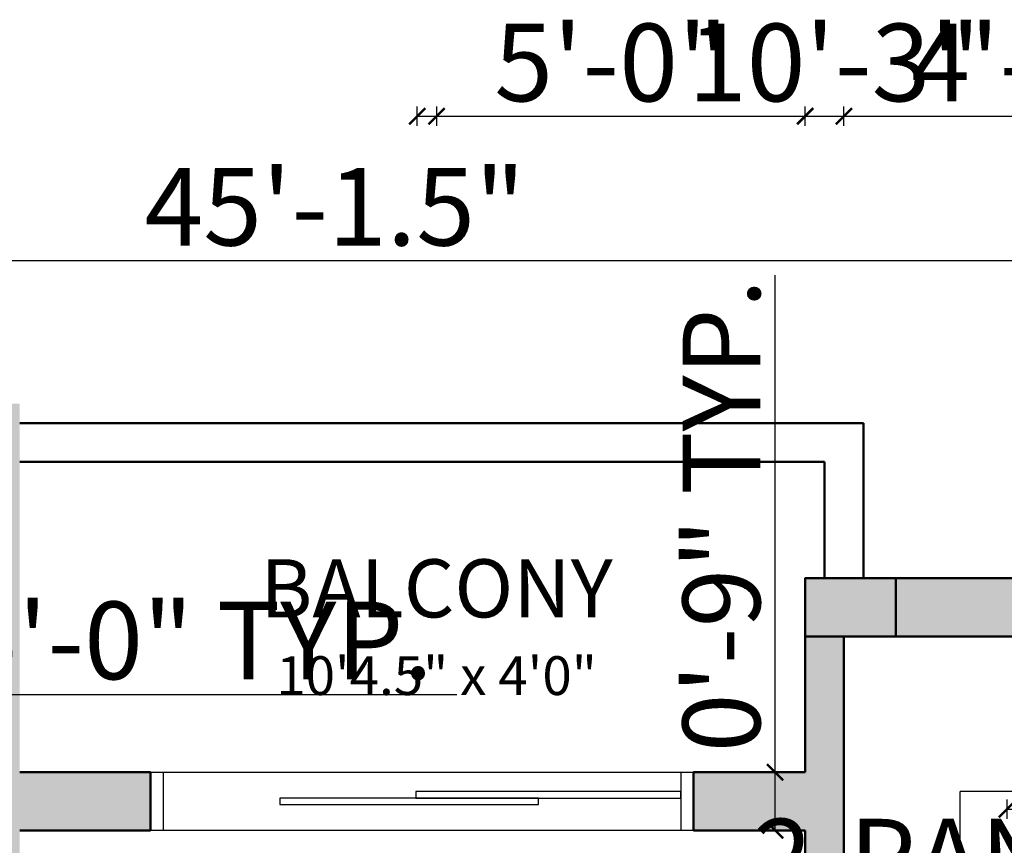
# Model space of a CAD drawing. Units: inches. Extents: x 375 to 1122, y 27 to 1069.
# Tile 150 of 155: x 667 to 819, y 941 to 1069. Entities that reach past the tile are written whole.
import ezdxf

# ---------------------------------------------------------------- set-up
doc = ezdxf.new("R2010")
doc.units = ezdxf.units.IN
for name, color, linetype, lineweight in [('A-ANNO-DIMS', 2, 'Continuous', 18), ('A-AREA-IDEN', 7, 'Continuous', 18), ('A-COLS-PATT', 10, 'Continuous', 13), ('A-FLOR-MILL', 55, 'Continuous', 25), ('A-WALL-PATT', 252, 'Continuous', 13), ('Columns', 10, 'Continuous', 50), ('Doors', 150, 'Continuous', 25), ('Walls', 250, 'Continuous', 50)]:
    doc.layers.add(name, color=color, linetype=linetype, lineweight=lineweight)
doc.styles.get("Standard").update_dxf_attribs({"font": 'arial.ttf'})
doc.dimstyles.new('ISO-25', dxfattribs={"dimtxt": 12, "dimasz": 2.5, "dimexe": 1.5, "dimexo": 1.5, "dimtad": 1, "dimdec": 1, "dimlunit": 3, "dimtxsty": 'Standard', "dimblk": 'ARCHTICK', "dimcen": 2.5, "dimadec": 0, "dimazin": 0, "dimtfac": 1, "dimtdec": 1, "dimtmove": 0, "dimatfit": 3, "dimfxl": 1.5, "dimfxlon": 1, "dimarcsym": 0})

# ---------------------------------------------------------------- blocks, each defined once
blk = doc.blocks.new('_ArchTick')
at = {"color": 0, "linetype": 'ByBlock', "const_width": 0.15}
blk.add_lwpolyline([(-0.5, -0.5), (0.5, 0.5)], dxfattribs=at)
blk = doc.blocks.new('*D27')
at = {"layer": 'A-ANNO-DIMS', "color": 0, "lineweight": -2, "transparency": 16777216}
for p, q in [((444.51, 1030.21), (444.51, 1033.21)), ((986.01, 1030.21), (986.01, 1033.21)), ((444.51, 1031.71), (986.01, 1031.71))]:
    blk.add_line(p, q, dxfattribs=at)
at = {"layer": 'Defpoints', "color": 0, "transparency": 16777216}
for p in [(986.01, 1031.71), (444.51, 982.53), (986.01, 982.53)]:
    blk.add_point(p, dxfattribs=at)
at = {"layer": 'A-ANNO-DIMS', "color": 0, "lineweight": -2, "transparency": 16777216, "xscale": 2.5, "yscale": 2.5, "zscale": 2.5, "rotation": 180}
blk.add_blockref('_ArchTick', (444.51, 1031.71), dxfattribs=at)
at = {"layer": 'A-ANNO-DIMS', "color": 0, "lineweight": -2, "transparency": 16777216, "xscale": 2.5, "yscale": 2.5, "zscale": 2.5}
blk.add_blockref('_ArchTick', (986.01, 1031.71), dxfattribs=at)
at = {"layer": 'A-ANNO-DIMS', "color": 0, "transparency": 16777216, "insert": (715.26, 1038.46), "char_height": 12, "attachment_point": 5}
blk.add_mtext('45\'-1.5"', dxfattribs=at)
blk = doc.blocks.new('BALCONY-SLIDER-2P-84IN')
for points in [[(0, 9), (84, 9), (84, 0), (0, 0)], [(20, 4), (60, 4), (60, 5), (20, 5)], [(41, 5), (82, 5), (82, 6), (41, 6)]]:
    blk.add_lwpolyline(points, close=True)
for points in [[(2, 0), (2, 9)], [(82, 9), (82, 0)]]:
    blk.add_lwpolyline(points)
blk = doc.blocks.new('COLUMN-14X9IN')
blk.add_lwpolyline([(0, 0), (14, 0), (14, 9), (0, 9)], close=True)
blk = doc.blocks.new('KITCHEN-COUNTER-L')
for p, q in [((0, 9), (0, 42)), ((87, 42), (0, 42)), ((87, 0), (87, 42)), ((87, 0), (111, 0))]:
    blk.add_line(p, q)
blk = doc.blocks.new('*D55')
at = {"layer": 'A-ANNO-DIMS', "color": 0, "lineweight": -2, "transparency": 16777216}
for p, q in [((518.51, 966.03), (518.51, 963.03)), ((578.51, 966.03), (578.51, 963.03)), ((518.51, 964.53), (578.51, 964.53)), ((578.51, 964.53), (734.11, 964.53))]:
    blk.add_line(p, q, dxfattribs=at)
at = {"layer": 'Defpoints', "color": 0, "transparency": 16777216}
for p in [(518.51, 973.53), (578.51, 973.53), (578.51, 964.53)]:
    blk.add_point(p, dxfattribs=at)
at = {"layer": 'A-ANNO-DIMS', "color": 0, "lineweight": -2, "transparency": 16777216, "xscale": 2.5, "yscale": 2.5, "zscale": 2.5, "rotation": 180}
blk.add_blockref('_ArchTick', (518.51, 964.53), dxfattribs=at)
at = {"layer": 'A-ANNO-DIMS', "color": 0, "lineweight": -2, "transparency": 16777216, "xscale": 2.5, "yscale": 2.5, "zscale": 2.5}
blk.add_blockref('_ArchTick', (578.51, 964.53), dxfattribs=at)
at = {"layer": 'A-ANNO-DIMS', "color": 0, "transparency": 16777216, "insert": (657.56, 971.36), "char_height": 12, "attachment_point": 5}
blk.add_mtext('WINDOW 5\'-0" TYP.', dxfattribs=at)
blk = doc.blocks.new('*D67')
at = {"layer": 'A-ANNO-DIMS', "color": 0, "lineweight": -2, "transparency": 16777216}
for p, q in [((819.23, 948.29), (819.23, 945.29)), ((853.33, 948.29), (853.33, 945.29)), ((819.23, 946.79), (853.33, 946.79)), ((853.33, 946.79), (1027.89, 946.79))]:
    blk.add_line(p, q, dxfattribs=at)
at = {"layer": 'Defpoints', "color": 0, "transparency": 16777216}
for p in [(819.23, 951.91), (853.33, 951.91), (853.33, 946.79)]:
    blk.add_point(p, dxfattribs=at)
at = {"layer": 'A-ANNO-DIMS', "color": 0, "lineweight": -2, "transparency": 16777216, "xscale": 2.5, "yscale": 2.5, "zscale": 2.5, "rotation": 180}
blk.add_blockref('_ArchTick', (819.23, 946.79), dxfattribs=at)
at = {"layer": 'A-ANNO-DIMS', "color": 0, "lineweight": -2, "transparency": 16777216, "xscale": 2.5, "yscale": 2.5, "zscale": 2.5}
blk.add_blockref('_ArchTick', (853.33, 946.79), dxfattribs=at)
at = {"layer": 'A-ANNO-DIMS', "color": 0, "transparency": 16777216, "insert": (941.86, 953.63), "char_height": 12, "attachment_point": 5}
blk.add_mtext('COOKTOP 2\'-10" TYP.', dxfattribs=at)
blk = doc.blocks.new('*D73')
at = {"layer": 'A-ANNO-DIMS', "color": 0, "lineweight": -2, "transparency": 16777216}
for p, q in [((686.76, 932.43), (686.76, 929.43)), ((770.76, 932.43), (770.76, 929.43)), ((686.76, 930.93), (770.76, 930.93)), ((770.76, 930.93), (987.61, 930.93))]:
    blk.add_line(p, q, dxfattribs=at)
at = {"layer": 'Defpoints', "color": 0, "transparency": 16777216}
for p in [(686.76, 943.53), (770.76, 943.53), (770.76, 930.93)]:
    blk.add_point(p, dxfattribs=at)
at = {"layer": 'A-ANNO-DIMS', "color": 0, "lineweight": -2, "transparency": 16777216, "xscale": 2.5, "yscale": 2.5, "zscale": 2.5, "rotation": 180}
blk.add_blockref('_ArchTick', (686.76, 930.93), dxfattribs=at)
at = {"layer": 'A-ANNO-DIMS', "color": 0, "lineweight": -2, "transparency": 16777216, "xscale": 2.5, "yscale": 2.5, "zscale": 2.5}
blk.add_blockref('_ArchTick', (770.76, 930.93), dxfattribs=at)
at = {"layer": 'A-ANNO-DIMS', "color": 0, "transparency": 16777216, "insert": (880.43, 937.76), "char_height": 12, "attachment_point": 5}
blk.add_mtext('2-PANEL SLIDER 7\'-0" TYP.', dxfattribs=at)
blk = doc.blocks.new('*D74')
at = {"layer": 'A-ANNO-DIMS', "color": 0, "lineweight": -2, "transparency": 16777216}
for p, q in [((783.36, 952.53), (783.36, 1029.42)), ((781.86, 952.53), (784.86, 952.53)), ((783.36, 943.53), (783.36, 952.53)), ((781.86, 943.53), (784.86, 943.53))]:
    blk.add_line(p, q, dxfattribs=at)
at = {"layer": 'Defpoints', "color": 0, "transparency": 16777216}
for p in [(770.76, 952.53), (783.36, 952.53), (770.76, 943.53)]:
    blk.add_point(p, dxfattribs=at)
at = {"layer": 'A-ANNO-DIMS', "color": 0, "lineweight": -2, "transparency": 16777216, "xscale": 2.5, "yscale": 2.5, "zscale": 2.5}
for p, rotation in [((783.36, 952.53), 90), ((783.36, 943.53), 270)]:
    blk.add_blockref('_ArchTick', p, dxfattribs=dict(at, rotation=rotation))
at = {"layer": 'A-ANNO-DIMS', "color": 0, "transparency": 16777216, "insert": (776.61, 992.23), "char_height": 12, "attachment_point": 5, "rotation": 90}
blk.add_mtext('0\'-9" TYP.', dxfattribs=at)
blk = doc.blocks.new('*D88')
at = {"layer": 'A-ANNO-DIMS', "color": 0, "lineweight": -2, "transparency": 16777216}
for p, q in [((731.01, 1052.53), (731.01, 1055.53)), ((854.01, 1052.53), (854.01, 1055.53)), ((731.01, 1054.03), (854.01, 1054.03))]:
    blk.add_line(p, q, dxfattribs=at)
at = {"layer": 'Defpoints', "color": 0, "transparency": 16777216}
for p in [(854.01, 1054.03), (731.01, 502.53), (854.01, 502.53)]:
    blk.add_point(p, dxfattribs=at)
at = {"layer": 'A-ANNO-DIMS', "color": 0, "lineweight": -2, "transparency": 16777216, "xscale": 2.5, "yscale": 2.5, "zscale": 2.5, "rotation": 180}
blk.add_blockref('_ArchTick', (731.01, 1054.03), dxfattribs=at)
at = {"layer": 'A-ANNO-DIMS', "color": 0, "lineweight": -2, "transparency": 16777216, "xscale": 2.5, "yscale": 2.5, "zscale": 2.5}
blk.add_blockref('_ArchTick', (854.01, 1054.03), dxfattribs=at)
at = {"layer": 'A-ANNO-DIMS', "color": 0, "transparency": 16777216, "insert": (792.51, 1060.78), "char_height": 12, "attachment_point": 5}
blk.add_mtext('10\'-3"', dxfattribs=at)
blk = doc.blocks.new('*D91')
at = {"layer": 'A-ANNO-DIMS', "color": 0, "lineweight": -2, "transparency": 16777216}
for p, q in [((728.01, 1052.53), (728.01, 1055.53)), ((788.01, 1052.53), (788.01, 1055.53)), ((728.01, 1054.03), (788.01, 1054.03))]:
    blk.add_line(p, q, dxfattribs=at)
at = {"layer": 'Defpoints', "color": 0, "transparency": 16777216}
for p in [(788.01, 1054.03), (728.01, 774.03), (788.01, 774.03)]:
    blk.add_point(p, dxfattribs=at)
at = {"layer": 'A-ANNO-DIMS', "color": 0, "lineweight": -2, "transparency": 16777216, "xscale": 2.5, "yscale": 2.5, "zscale": 2.5, "rotation": 180}
blk.add_blockref('_ArchTick', (728.01, 1054.03), dxfattribs=at)
at = {"layer": 'A-ANNO-DIMS', "color": 0, "lineweight": -2, "transparency": 16777216, "xscale": 2.5, "yscale": 2.5, "zscale": 2.5}
blk.add_blockref('_ArchTick', (788.01, 1054.03), dxfattribs=at)
at = {"layer": 'A-ANNO-DIMS', "color": 0, "transparency": 16777216, "insert": (758.01, 1060.78), "char_height": 12, "attachment_point": 5}
blk.add_mtext('5\'-0"', dxfattribs=at)
blk = doc.blocks.new('*D96')
at = {"layer": 'A-ANNO-DIMS', "color": 0, "lineweight": -2, "transparency": 16777216}
for p, q in [((794.01, 1052.53), (794.01, 1055.53)), ((851.01, 1052.53), (851.01, 1055.53)), ((794.01, 1054.03), (851.01, 1054.03))]:
    blk.add_line(p, q, dxfattribs=at)
at = {"layer": 'Defpoints', "color": 0, "transparency": 16777216}
for p in [(851.01, 1054.03), (794.01, 973.53), (851.01, 973.53)]:
    blk.add_point(p, dxfattribs=at)
at = {"layer": 'A-ANNO-DIMS', "color": 0, "lineweight": -2, "transparency": 16777216, "xscale": 2.5, "yscale": 2.5, "zscale": 2.5, "rotation": 180}
blk.add_blockref('_ArchTick', (794.01, 1054.03), dxfattribs=at)
at = {"layer": 'A-ANNO-DIMS', "color": 0, "lineweight": -2, "transparency": 16777216, "xscale": 2.5, "yscale": 2.5, "zscale": 2.5}
blk.add_blockref('_ArchTick', (851.01, 1054.03), dxfattribs=at)
at = {"layer": 'A-ANNO-DIMS', "color": 0, "transparency": 16777216, "insert": (822.51, 1060.78), "char_height": 12, "attachment_point": 5}
blk.add_mtext('4\'-9"', dxfattribs=at)

msp = doc.modelspace()

# ---------------------------------------------------------------- hatches: boundary and pattern name
at = {"layer": 'A-COLS-PATT'}
h = msp.add_hatch(color=256, dxfattribs=at)
h.dxf.hatch_style = 1
h.paths.add_polyline_path([(512.51, 982.53), (498.51, 982.53), (498.51, 973.53), (512.51, 973.53)])
h.paths.add_polyline_path([(666.51, 982.53), (652.51, 982.53), (652.51, 973.53), (666.51, 973.53)])
h.paths.add_polyline_path([(802.01, 982.53), (788.01, 982.53), (788.01, 973.53), (802.01, 973.53)])
h.paths.add_polyline_path([(932.01, 982.53), (918.01, 982.53), (918.01, 973.53), (932.01, 973.53)])
h.paths.add_polyline_path([(507.51, 841.53), (498.51, 841.53), (498.51, 827.53), (507.51, 827.53)])
h.paths.add_polyline_path([(666.51, 844.53), (652.51, 844.53), (652.51, 835.53), (666.51, 835.53)])
h.paths.add_polyline_path([(802.01, 814.53), (788.01, 814.53), (788.01, 805.53), (802.01, 805.53)])
h.paths.add_polyline_path([(932.01, 814.53), (918.01, 814.53), (918.01, 805.53), (932.01, 805.53)])
h.paths.add_polyline_path([(507.51, 719.53), (498.51, 719.53), (498.51, 705.53), (507.51, 705.53)])
h.paths.add_polyline_path([(731.01, 676.53), (722.01, 676.53), (722.01, 662.53), (731.01, 662.53)])
h.paths.add_polyline_path([(802.01, 676.53), (788.01, 676.53), (788.01, 667.53), (802.01, 667.53)])
h.paths.add_polyline_path([(932.01, 676.53), (918.01, 676.53), (918.01, 667.53), (932.01, 667.53)])
h.paths.add_polyline_path([(932.01, 583.53), (918.01, 583.53), (918.01, 574.53), (932.01, 574.53)])
h.paths.add_polyline_path([(868.01, 583.53), (854.01, 583.53), (854.01, 574.53), (868.01, 574.53)])
h.paths.add_polyline_path([(868.01, 502.53), (854.01, 502.53), (854.01, 493.53), (868.01, 493.53)])
h.paths.add_polyline_path([(932.01, 502.53), (918.01, 502.53), (918.01, 493.53), (932.01, 493.53)])
h.paths.add_polyline_path([(672.51, 592.03), (663.51, 592.03), (663.51, 578.03), (672.51, 578.03)])
h.paths.add_polyline_path([(512.51, 589.53), (498.51, 589.53), (498.51, 580.53), (512.51, 580.53)])
h.paths.add_polyline_path([(507.51, 464.53), (498.51, 464.53), (498.51, 450.53), (507.51, 450.53)])
h.paths.add_polyline_path([(731.01, 507.53), (722.01, 507.53), (722.01, 493.53), (731.01, 493.53)])
h.paths.add_polyline_path([(802.01, 502.53), (788.01, 502.53), (788.01, 493.53), (802.01, 493.53)])
h.paths.add_polyline_path([(507.51, 342.53), (498.51, 342.53), (498.51, 328.53), (507.51, 328.53)])
h.paths.add_polyline_path([(512.51, 196.53), (498.51, 196.53), (498.51, 187.53), (512.51, 187.53)])
h.paths.add_polyline_path([(666.51, 334.53), (652.51, 334.53), (652.51, 325.53), (666.51, 325.53)])
h.paths.add_polyline_path([(666.51, 196.53), (652.51, 196.53), (652.51, 187.53), (666.51, 187.53)])
h.paths.add_polyline_path([(805.01, 196.53), (791.01, 196.53), (791.01, 187.53), (805.01, 187.53)])
h.paths.add_polyline_path([(932.01, 196.53), (918.01, 196.53), (918.01, 187.53), (932.01, 187.53)])
h.paths.add_polyline_path([(932.01, 334.53), (918.01, 334.53), (918.01, 325.53), (932.01, 325.53)])
h.paths.add_polyline_path([(805.01, 334.53), (791.01, 334.53), (791.01, 325.53), (805.01, 325.53)])
at = {"layer": 'A-WALL-PATT'}
h = msp.add_hatch(color=256, dxfattribs=at)
h.dxf.hatch_style = 1
h.paths.add_polyline_path([(962.01, 388.53), (989.01, 388.53), (989.01, 394.53), (962.01, 394.53), (932.01, 394.53), (932.01, 397.53), (923.01, 397.53), (923.01, 394.53), (842.01, 394.53), (842.01, 334.53), (839.51, 334.53), (839.51, 328.53), (854.01, 328.53), (854.01, 334.53), (848.01, 334.53), (848.01, 388.53), (953.01, 388.53), (953.01, 356.08), (962.01, 356.08), (962.01, 358.55), (989.01, 358.55), (989.01, 364.55), (962.01, 364.55)])
h.paths.add_polyline_path([(989.01, 502.53), (932.01, 502.53), (932.01, 583.53), (932.01, 593.53), (923.01, 593.53), (923.01, 583.53), (854.01, 583.53), (854.01, 556.53), (863.01, 556.53), (863.01, 574.53), (923.01, 574.53), (923.01, 502.53), (863.01, 502.53), (863.01, 520.53), (854.01, 520.53), (854.01, 502.53), (773.01, 502.53), (773.01, 493.53), (788.01, 493.53), (788.01, 402.03), (722.01, 402.03), (722.01, 373.53), (728.01, 373.53), (728.01, 396.03), (788.01, 396.03), (788.01, 373.53), (794.01, 373.53), (794.01, 430.53), (814.01, 430.53), (814.01, 436.53), (794.01, 436.53), (794.01, 493.53), (923.01, 493.53), (923.01, 487.53), (932.01, 487.53), (932.01, 493.53), (983.01, 493.53), (983.01, 473.53), (989.01, 473.53)])
h.paths.add_polyline_path([(797.01, 325.53), (805.01, 325.53), (805.01, 328.53), (807.51, 328.53), (807.51, 334.53), (791.01, 334.53), (791.01, 226.53), (770.76, 226.53), (770.76, 217.53), (791.01, 217.53), (791.01, 187.53), (855.01, 187.53), (855.01, 196.53), (797.01, 196.53)])
h.paths.add_polyline_path([(989.01, 238.53), (962.01, 238.53), (962.01, 256.42), (953.01, 256.42), (953.01, 229.53), (980.01, 229.53), (980.01, 196.53), (915.01, 196.53), (915.01, 187.53), (989.01, 187.53)])
h.paths.add_polyline_path([(962.01, 334.53), (884.01, 334.53), (884.01, 328.53), (918.01, 328.53), (918.01, 325.53), (932.01, 325.53), (932.01, 328.53), (953.01, 328.53), (953.01, 304.42), (962.01, 304.42)])
h.paths.add_polyline_path([(606.51, 283.53), (609.51, 283.53), (609.51, 289.53), (600.51, 289.53), (600.51, 196.53), (578.51, 196.53), (578.51, 187.53), (606.51, 187.53), (606.51, 196.53)])
h.paths.add_polyline_path([(666.51, 292.53), (660.51, 292.53), (660.51, 289.53), (633.51, 289.53), (633.51, 283.53), (660.51, 283.53), (660.51, 196.53), (628.01, 196.53), (628.01, 187.53), (630.53, 187.53), (630.53, 160.53), (636.53, 160.53), (636.53, 187.53), (660.51, 187.53), (660.51, 160.53), (666.51, 160.53), (666.51, 217.53), (686.76, 217.53), (686.76, 226.53), (666.51, 226.53)])
h.paths.add_polyline_path([(480.51, 256.42), (471.51, 256.42), (471.51, 238.53), (444.51, 238.53), (444.51, 187.53), (518.51, 187.53), (518.51, 196.53), (453.51, 196.53), (453.51, 229.53), (480.51, 229.53)])
h.paths.add_polyline_path([(480.51, 328.53), (652.51, 328.53), (652.51, 325.53), (660.51, 325.53), (660.51, 322.53), (666.51, 322.53), (666.51, 334.53), (507.51, 334.53), (507.51, 360.53), (498.51, 360.53), (498.51, 334.53), (471.51, 334.53), (471.51, 304.42), (480.51, 304.42)])
h.paths.add_polyline_path([(507.51, 484.53), (498.51, 484.53), (498.51, 444.53), (507.51, 444.53), (507.51, 454.53), (621.51, 454.53), (621.51, 460.53), (507.51, 460.53)])
h.paths.add_polyline_path([(672.51, 604.53), (683.26, 604.53), (683.26, 613.53), (669.51, 613.53), (669.51, 649.53), (663.51, 649.53), (663.51, 589.53), (507.51, 589.53), (507.51, 613.53), (498.51, 613.53), (498.51, 556.53), (507.51, 556.53), (507.51, 580.53), (663.51, 580.53), (663.51, 520.53), (669.51, 520.53), (669.51, 556.53), (683.26, 556.53), (683.26, 565.53), (672.51, 565.53)])
h.paths.add_polyline_path([(731.01, 667.53), (734.01, 667.53), (734.01, 676.53), (728.01, 676.53), (728.01, 715.53), (657.51, 715.53), (657.51, 709.53), (663.51, 709.53), (663.51, 673.53), (669.51, 673.53), (669.51, 709.53), (722.01, 709.53), (722.01, 613.53), (704.76, 613.53), (704.76, 604.53), (722.01, 604.53), (722.01, 565.53), (704.76, 565.53), (704.76, 556.53), (722.01, 556.53), (722.01, 502.53), (722.01, 460.53), (669.51, 460.53), (669.51, 496.53), (663.51, 496.53), (663.51, 460.53), (657.51, 460.53), (657.51, 454.53), (728.01, 454.53), (728.01, 493.53), (734.01, 493.53), (734.01, 502.53), (731.01, 502.53)])
h.paths.add_polyline_path([(986.01, 718.53), (959.01, 718.53), (959.01, 727.53), (950.01, 727.53), (950.01, 709.53), (977.01, 709.53), (977.01, 676.53), (794.01, 676.53), (794.01, 805.53), (802.01, 805.53), (802.01, 808.53), (804.51, 808.53), (804.51, 814.53), (788.01, 814.53), (788.01, 774.03), (728.01, 774.03), (728.01, 796.53), (722.01, 796.53), (722.01, 768.03), (788.01, 768.03), (788.01, 676.53), (773.01, 676.53), (773.01, 667.53), (923.01, 667.53), (923.01, 657.53), (932.01, 657.53), (932.01, 667.53), (986.01, 667.53)])
h.paths.add_polyline_path([(621.51, 715.53), (507.51, 715.53), (507.51, 733.53), (498.51, 733.53), (498.51, 715.53), (498.51, 685.53), (507.51, 685.53), (507.51, 709.53), (621.51, 709.53)])
h.paths.add_polyline_path([(666.51, 847.03), (660.51, 847.03), (660.51, 844.53), (652.51, 844.53), (652.51, 841.53), (480.51, 841.53), (480.51, 859.53), (471.51, 859.53), (471.51, 835.53), (498.51, 835.53), (498.51, 817.53), (507.51, 817.53), (507.51, 835.53), (666.51, 835.53)])
h.paths.add_polyline_path([(480.51, 940.53), (453.51, 940.53), (453.51, 973.53), (518.51, 973.53), (518.51, 982.53), (444.51, 982.53), (444.51, 931.53), (471.51, 931.53), (471.51, 907.53), (480.51, 907.53)])
h.paths.add_polyline_path([(606.51, 982.53), (578.51, 982.53), (578.51, 973.53), (600.51, 973.53), (600.51, 880.53), (609.51, 880.53), (609.51, 886.53), (606.51, 886.53)])
h.paths.add_polyline_path([(666.51, 943.53), (686.76, 943.53), (686.76, 952.53), (666.51, 952.53), (666.51, 1009.53), (660.51, 1009.53), (660.51, 982.53), (636.53, 982.53), (636.53, 1009.53), (630.53, 1009.53), (630.53, 982.53), (628.01, 982.53), (628.01, 973.53), (660.51, 973.53), (660.51, 886.53), (633.51, 886.53), (633.51, 880.53), (660.51, 880.53), (660.51, 877.03), (666.51, 877.03)])
h.paths.add_polyline_path([(986.01, 874.53), (932.01, 874.53), (932.01, 877.53), (923.01, 877.53), (923.01, 874.53), (788.01, 874.53), (788.01, 868.53), (788.01, 844.53), (794.01, 844.53), (794.01, 868.53), (839.01, 868.53), (839.01, 814.53), (836.51, 814.53), (836.51, 808.53), (851.01, 808.53), (851.01, 814.53), (845.01, 814.53), (845.01, 868.53), (986.01, 868.53)])
h.paths.add_polyline_path([(959.01, 838.55), (986.01, 838.55), (986.01, 844.55), (959.01, 844.55), (959.01, 847.03), (950.01, 847.03), (950.01, 814.53), (881.01, 814.53), (881.01, 808.53), (918.01, 808.53), (918.01, 805.53), (932.01, 805.53), (932.01, 808.53), (950.01, 808.53), (950.01, 793.53), (959.01, 793.53)])
h.paths.add_polyline_path([(986.01, 982.53), (899.01, 982.53), (899.01, 973.53), (923.01, 973.53), (923.01, 967.53), (932.01, 967.53), (932.01, 973.53), (980.01, 973.53), (980.01, 953.53), (986.01, 953.53)])
h.paths.add_polyline_path([(851.01, 982.53), (788.01, 982.53), (788.01, 952.53), (770.76, 952.53), (770.76, 943.53), (788.01, 943.53), (788.01, 910.53), (814.01, 910.53), (814.01, 916.53), (794.01, 916.53), (794.01, 973.53), (851.01, 973.53)])

# ---------------------------------------------------------------- linework, layer by layer
at = {"layer": 'Walls'}
for p, q in [((797.01, 1006.53), (666.51, 1006.53)), ((797.01, 1006.53), (797.01, 982.53)), ((791.01, 1000.53), (666.51, 1000.53)), ((791.01, 982.53), (791.01, 1000.53)), ((788.01, 952.53), (788.01, 982.53)), ((851.01, 982.53), (788.01, 982.53)), ((794.01, 916.53), (794.01, 973.53)), ((851.01, 973.53), (794.01, 973.53)), ((686.76, 952.53), (666.51, 952.53)), ((686.76, 943.53), (686.76, 952.53)), ((788.01, 952.53), (770.76, 952.53)), ((770.76, 943.53), (770.76, 952.53)), ((686.76, 943.53), (666.51, 943.53)), ((788.01, 943.53), (770.76, 943.53)), ((788.01, 910.53), (788.01, 943.53))]:
    msp.add_line(p, q, dxfattribs=at)

# ---------------------------------------------------------------- block references
at = {"layer": 'A-FLOR-MILL'}
msp.add_blockref('KITCHEN-COUNTER-L', (812.01, 907.53), dxfattribs=at)
at = {"layer": 'Columns', "rotation": 180}
msp.add_blockref('COLUMN-14X9IN', (802.01, 982.53), dxfattribs=at)
at = {"layer": 'Doors'}
msp.add_blockref('BALCONY-SLIDER-2P-84IN', (686.76, 943.53), dxfattribs=at)

# ---------------------------------------------------------------- texts
at = {"layer": 'A-AREA-IDEN', "insert": (697.93, 964.47), "char_height": 12, "attachment_point": 7}
msp.add_mtext_dynamic_manual_height_columns('\\pxqc;{\\fArial|b1|i0|c0|p34;\\H0.75x;BALCONY\\H1.33333x;\\P\\fArial|b0|i0|c0|p34;\\H0.5x;10\'4.5" x 4\'0"}', width=66.1169, gutter_width=12.5, heights=[0], dxfattribs=at)

# ---------------------------------------------------------------- dimensions: what is measured, and where the dimension line sits
at = {"layer": 'A-ANNO-DIMS'}
for base, p1, p2, picture, middle in [((788.01, 1054.03), (728.01, 774.03), (788.01, 774.03), '*D91', (758.01, 1060.78)), ((854.01, 1054.03), (731.01, 502.53), (854.01, 502.53), '*D88', (792.51, 1060.78)), ((851.01, 1054.03), (794.01, 973.53), (851.01, 973.53), '*D96', (822.51, 1060.78))]:
    dim = msp.add_linear_dim(base=base, p1=p1, p2=p2, dimstyle='ISO-25', override={"dimdec": 1, "dimlfac": 1, "dimrnd": 0, "dimzin": 1, "dimdsep": 46, "dimlunit": 4, "dimfrac": 2}, dxfattribs=at)
    dim.commit()
    dim.dimension.update_dxf_attribs({"geometry": picture, "text_midpoint": middle})
dim = msp.add_linear_dim(base=(986.01, 1031.71), p1=(444.51, 982.53), p2=(986.01, 982.53), dimstyle='ISO-25', override={"dimclrd": 0, "dimclre": 0, "dimclrt": 0}, dxfattribs=at)
dim.commit()
dim.dimension.update_dxf_attribs({"geometry": '*D27', "text_midpoint": (715.26, 1031.71), "dimtype": 160})
dim = msp.add_linear_dim(base=(783.36, 952.53), p1=(770.76, 943.53), p2=(770.76, 952.53), angle=90, text='<> TYP.', dimstyle='ISO-25', override={"dimdec": 1, "dimlfac": 1, "dimrnd": 0, "dimzin": 1, "dimdsep": 46, "dimlunit": 4, "dimfrac": 2}, dxfattribs=at)
dim.commit()
dim.dimension.update_dxf_attribs({"geometry": '*D74', "text_midpoint": (776.61, 992.23)})
for base, p1, p2, text, picture, middle in [((578.51, 964.53), (518.51, 973.53), (578.51, 973.53), 'WINDOW <> TYP.', '*D55', (657.56, 971.36)), ((853.33, 946.79), (819.23, 951.91), (853.33, 951.91), 'COOKTOP <> TYP.', '*D67', (941.86, 953.63)), ((770.76, 930.93), (686.76, 943.53), (770.76, 943.53), '2-PANEL SLIDER <> TYP.', '*D73', (880.43, 937.76))]:
    dim = msp.add_linear_dim(base=base, p1=p1, p2=p2, text=text, dimstyle='ISO-25', override={"dimdec": 1, "dimlfac": 1, "dimrnd": 0, "dimzin": 1, "dimdsep": 46, "dimlunit": 4, "dimfrac": 2}, dxfattribs=at)
    dim.commit()
    dim.dimension.update_dxf_attribs({"geometry": picture, "text_midpoint": middle})

doc.saveas('drawing.dxf')
